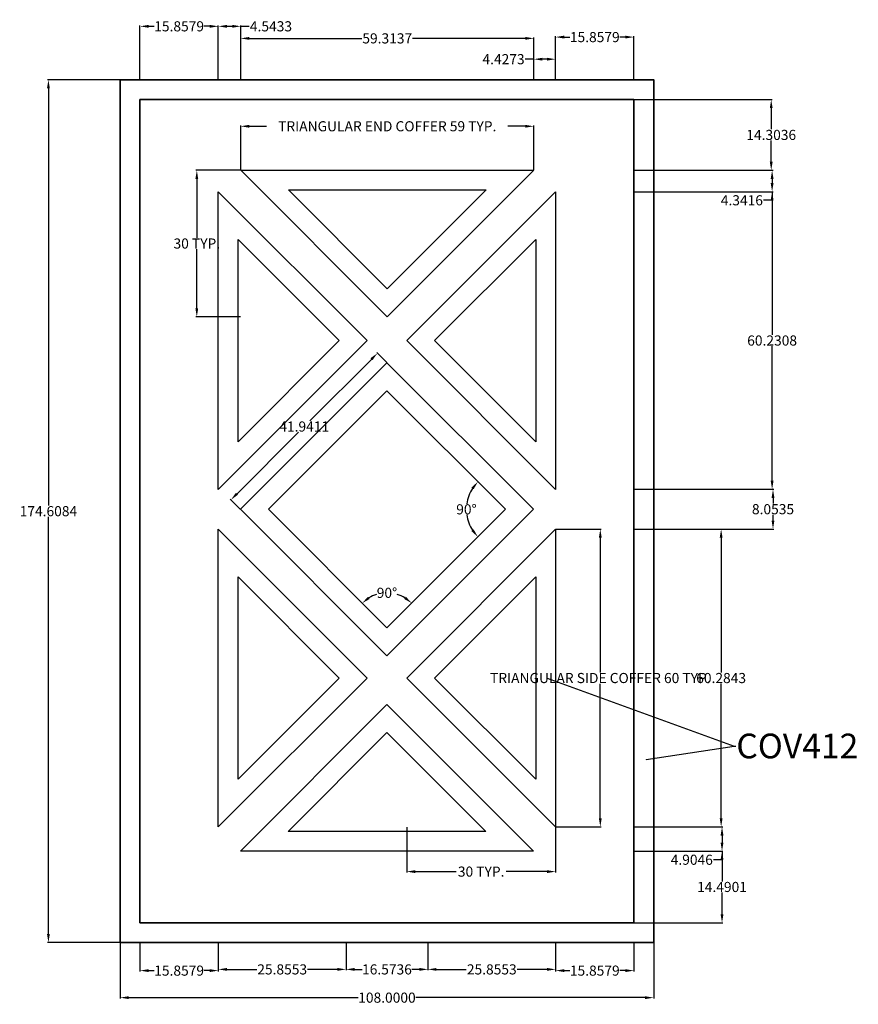
# Model space of a CAD drawing. Units: inches. Extents: x 854 to 1024, y 578 to 778.
import ezdxf
from ezdxf import colors
from ezdxf.entities.mleader import LeaderData, LeaderLine
from ezdxf.math import Vec2, Vec3

# ---------------------------------------------------------------- set-up
doc = ezdxf.new("R2010")
doc.units = ezdxf.units.IN
doc.header["$MEASUREMENT"] = 0
for name, color, linetype, lineweight in [('A-ANNO-DIMS', 2, 'Continuous', 18), ('A-ANNO-TEXT', 3, 'Continuous', 18), ('A-CLNG', 7, 'Continuous', 35), ('A-CLNG-COFR', 4, 'Continuous', 25)]:
    doc.layers.add(name, color=color, linetype=linetype, lineweight=lineweight)
doc.styles.get("Standard").update_dxf_attribs({"font": 'arial.ttf'})
doc.dimstyles.get("Standard").update_dxf_attribs({"dimtxt": 2.0485, "dimasz": 1.737, "dimexe": 0.18, "dimexo": 0.0625, "dimgap": 0.09, "dimtad": 0, "dimtih": 1, "dimtoh": 1, "dimdec": 4, "dimzin": 0, "dimdsep": 46, "dimtxsty": 'Standard', "dimcen": 0.09, "dimadec": 0, "dimazin": 0, "dimtfac": 1, "dimtdec": 4, "dimtofl": 0, "dimtmove": 0, "dimatfit": 3, "dimfxl": 1, "dimtolj": 1, "dimtzin": 0, "dimarcsym": 0})

# ---------------------------------------------------------------- blocks, each defined once
blk = doc.blocks.new('*D1')
at = {"layer": 'A-ANNO-DIMS', "color": 0, "lineweight": -2, "transparency": 16777216}
for start, end in [(147.6108, 171.7413), (188.2587, 212.3892)]:
    blk.add_arc((952.75, 678.63), 7.91, start, end, dxfattribs=at)
at = {"layer": 'A-ANNO-DIMS', "color": 0, "transparency": 16777216}
for points in [[(945.85, 683.05), (946.3, 682.69), (947.16, 684.23)], [(946.3, 674.58), (945.85, 674.22), (947.16, 673.04)]]:
    blk.add_solid(points, dxfattribs=at)
at = {"layer": 'Defpoints', "color": 0, "transparency": 16777216}
for p in [(928.75, 702.63), (945.11, 680.68), (952.75, 678.63), (952.75, 678.63), (928.75, 654.63)]:
    blk.add_point(p, dxfattribs=at)
at = {"layer": 'A-ANNO-DIMS', "color": 0, "transparency": 16777216, "insert": (944.84, 678.63), "char_height": 2.049, "attachment_point": 5}
blk.add_mtext('\\A1;90°', dxfattribs=at)
blk = doc.blocks.new('*D2')
at = {"layer": 'A-ANNO-DIMS', "color": 0, "lineweight": -2, "transparency": 16777216}
for start, end in [(107.2, 120.9465), (59.0535, 72.8)]:
    blk.add_arc((928.75, 654.63), 7.1, start, end, dxfattribs=at)
at = {"layer": 'A-ANNO-DIMS', "color": 0, "transparency": 16777216}
for points in [[(925.28, 660.5), (924.92, 660.95), (923.73, 659.65)], [(932.58, 660.95), (932.22, 660.5), (933.77, 659.65)]]:
    blk.add_solid(points, dxfattribs=at)
at = {"layer": 'Defpoints', "color": 0, "transparency": 16777216}
for p in [(904.75, 678.63), (952.75, 678.63), (930.59, 661.49), (928.75, 654.63), (928.75, 654.63)]:
    blk.add_point(p, dxfattribs=at)
at = {"layer": 'A-ANNO-DIMS', "color": 0, "transparency": 16777216, "insert": (928.75, 661.73), "char_height": 2.049, "attachment_point": 5}
blk.add_mtext('\\A1;90°', dxfattribs=at)
blk = doc.blocks.new('*D3')
at = {"layer": 'A-ANNO-DIMS', "color": 0, "lineweight": -2, "transparency": 16777216}
for p, q in [((928.71, 708.34), (926.7, 710.35)), ((925.6, 708.99), (913.13, 696.53)), ((898.4, 681.79), (910.86, 694.25)), ((899.05, 678.68), (897.04, 680.69))]:
    blk.add_line(p, q, dxfattribs=at)
at = {"layer": 'A-ANNO-DIMS', "color": 0, "transparency": 16777216}
for points in [[(925.39, 709.2), (925.8, 708.79), (926.82, 710.22)], [(898.19, 682), (898.6, 681.59), (897.17, 680.56)]]:
    blk.add_solid(points, dxfattribs=at)
at = {"layer": 'Defpoints', "color": 0, "transparency": 16777216}
for p in [(926.82, 710.22), (928.75, 708.29), (899.09, 678.63)]:
    blk.add_point(p, dxfattribs=at)
at = {"layer": 'A-ANNO-DIMS', "color": 0, "transparency": 16777216, "insert": (912, 695.39), "char_height": 2.0485, "attachment_point": 5}
blk.add_mtext('\\A1;41.9411', dxfattribs=at)
blk = doc.blocks.new('*D4')
at = {"layer": 'A-ANNO-DIMS', "color": 0, "lineweight": -2, "transparency": 16777216}
for p, q in [((874.75, 590.89), (874.75, 579.62)), ((982.75, 590.89), (982.75, 579.62)), ((876.49, 579.8), (922.92, 579.8)), ((981.01, 579.8), (934.58, 579.8))]:
    blk.add_line(p, q, dxfattribs=at)
at = {"layer": 'A-ANNO-DIMS', "color": 0, "transparency": 16777216}
for points in [[(876.49, 580.09), (876.49, 579.51), (874.75, 579.8)], [(981.01, 580.09), (981.01, 579.51), (982.75, 579.8)]]:
    blk.add_solid(points, dxfattribs=at)
at = {"layer": 'Defpoints', "color": 0, "transparency": 16777216}
for p in [(874.75, 590.96), (982.75, 590.96), (982.75, 579.8)]:
    blk.add_point(p, dxfattribs=at)
at = {"layer": 'A-ANNO-DIMS', "color": 0, "transparency": 16777216, "insert": (928.75, 579.8), "char_height": 2.0485, "attachment_point": 5}
blk.add_mtext('\\A1;108.0000', dxfattribs=at)
blk = doc.blocks.new('*D5')
at = {"layer": 'A-ANNO-DIMS', "color": 0, "lineweight": -2, "transparency": 16777216}
for p, q in [((874.69, 765.56), (860.04, 765.56)), ((860.22, 763.83), (860.22, 679.4)), ((860.22, 592.69), (860.22, 677.12)), ((874.69, 590.96), (860.04, 590.96))]:
    blk.add_line(p, q, dxfattribs=at)
at = {"layer": 'A-ANNO-DIMS', "color": 0, "transparency": 16777216}
for points in [[(859.93, 763.83), (860.51, 763.83), (860.22, 765.56)], [(859.93, 592.69), (860.51, 592.69), (860.22, 590.96)]]:
    blk.add_solid(points, dxfattribs=at)
at = {"layer": 'Defpoints', "color": 0, "transparency": 16777216}
for p in [(874.75, 765.56), (860.22, 590.96), (874.75, 590.96)]:
    blk.add_point(p, dxfattribs=at)
at = {"layer": 'A-ANNO-DIMS', "color": 0, "transparency": 16777216, "insert": (860.22, 678.26), "char_height": 2.0485, "attachment_point": 5}
blk.add_mtext('\\A1;174.6084', dxfattribs=at)
blk = doc.blocks.new('*D6')
at = {"layer": 'A-ANNO-DIMS', "color": 0, "lineweight": -2, "transparency": 16777216}
for p, q in [((878.75, 765.63), (878.75, 776.57)), ((880.49, 776.39), (881.64, 776.39)), ((892.87, 776.39), (891.72, 776.39)), ((894.61, 765.63), (894.61, 776.57))]:
    blk.add_line(p, q, dxfattribs=at)
at = {"layer": 'A-ANNO-DIMS', "color": 0, "transparency": 16777216}
for points in [[(880.49, 776.68), (880.49, 776.1), (878.75, 776.39)], [(892.87, 776.68), (892.87, 776.1), (894.61, 776.39)]]:
    blk.add_solid(points, dxfattribs=at)
at = {"layer": 'Defpoints', "color": 0, "transparency": 16777216}
for p in [(894.61, 776.39), (878.75, 765.56), (894.61, 765.56)]:
    blk.add_point(p, dxfattribs=at)
at = {"layer": 'A-ANNO-DIMS', "color": 0, "transparency": 16777216, "insert": (886.68, 776.39), "char_height": 2.0485, "attachment_point": 5}
blk.add_mtext('\\A1;15.8579', dxfattribs=at)
blk = doc.blocks.new('*D7')
at = {"layer": 'A-ANNO-DIMS', "color": 0, "lineweight": -2, "transparency": 16777216}
for p, q in [((894.61, 765.63), (894.61, 776.57)), ((896.35, 776.39), (897.42, 776.39)), ((899.15, 765.63), (899.15, 776.57)), ((899.15, 776.39), (900.89, 776.39))]:
    blk.add_line(p, q, dxfattribs=at)
at = {"layer": 'A-ANNO-DIMS', "color": 0, "transparency": 16777216}
for points in [[(896.35, 776.68), (896.35, 776.1), (894.61, 776.39)], [(897.42, 776.68), (897.42, 776.1), (899.15, 776.39)]]:
    blk.add_solid(points, dxfattribs=at)
at = {"layer": 'Defpoints', "color": 0, "transparency": 16777216}
for p in [(899.15, 776.39), (894.61, 765.56), (899.15, 765.56)]:
    blk.add_point(p, dxfattribs=at)
at = {"layer": 'A-ANNO-DIMS', "color": 0, "transparency": 16777216, "insert": (905.27, 776.39), "char_height": 2.049, "attachment_point": 5}
blk.add_mtext('\\A1;4.5433', dxfattribs=at)
blk = doc.blocks.new('*D8')
at = {"layer": 'A-ANNO-DIMS', "color": 0, "lineweight": -2, "transparency": 16777216}
for p, q in [((899.15, 765.63), (899.15, 774.13)), ((900.89, 773.95), (923.67, 773.95)), ((956.73, 773.95), (933.95, 773.95)), ((958.47, 765.63), (958.47, 774.13))]:
    blk.add_line(p, q, dxfattribs=at)
at = {"layer": 'A-ANNO-DIMS', "color": 0, "transparency": 16777216}
for points in [[(900.89, 774.24), (900.89, 773.66), (899.15, 773.95)], [(956.73, 774.24), (956.73, 773.66), (958.47, 773.95)]]:
    blk.add_solid(points, dxfattribs=at)
at = {"layer": 'Defpoints', "color": 0, "transparency": 16777216}
for p in [(958.47, 773.95), (899.15, 765.56), (958.47, 765.56)]:
    blk.add_point(p, dxfattribs=at)
at = {"layer": 'A-ANNO-DIMS', "color": 0, "transparency": 16777216, "insert": (928.81, 773.95), "char_height": 2.0485, "attachment_point": 5}
blk.add_mtext('\\A1;59.3137', dxfattribs=at)
blk = doc.blocks.new('*D9')
at = {"layer": 'A-ANNO-DIMS', "color": 0, "lineweight": -2, "transparency": 16777216}
for p, q in [((958.47, 769.74), (956.73, 769.74)), ((958.47, 765.63), (958.47, 769.92)), ((961.16, 769.74), (960.2, 769.74)), ((962.89, 765.63), (962.89, 769.92))]:
    blk.add_line(p, q, dxfattribs=at)
at = {"layer": 'A-ANNO-DIMS', "color": 0, "transparency": 16777216}
for points in [[(960.2, 770.02), (960.2, 769.45), (958.47, 769.74)], [(961.16, 770.02), (961.16, 769.45), (962.89, 769.74)]]:
    blk.add_solid(points, dxfattribs=at)
at = {"layer": 'Defpoints', "color": 0, "transparency": 16777216}
for p in [(958.47, 769.74), (958.47, 765.56), (962.89, 765.56)]:
    blk.add_point(p, dxfattribs=at)
at = {"layer": 'A-ANNO-DIMS', "color": 0, "transparency": 16777216, "insert": (952.35, 769.74), "char_height": 2.049, "attachment_point": 5}
blk.add_mtext('\\A1;4.4273', dxfattribs=at)
blk = doc.blocks.new('*D10')
at = {"layer": 'A-ANNO-DIMS', "color": 0, "lineweight": -2, "transparency": 16777216}
for p, q in [((962.89, 765.63), (962.89, 774.39)), ((964.63, 774.21), (965.78, 774.21)), ((977.01, 774.21), (975.87, 774.21)), ((978.75, 765.63), (978.75, 774.39))]:
    blk.add_line(p, q, dxfattribs=at)
at = {"layer": 'A-ANNO-DIMS', "color": 0, "transparency": 16777216}
for points in [[(964.63, 774.5), (964.63, 773.92), (962.89, 774.21)], [(977.01, 774.5), (977.01, 773.92), (978.75, 774.21)]]:
    blk.add_solid(points, dxfattribs=at)
at = {"layer": 'Defpoints', "color": 0, "transparency": 16777216}
for p in [(978.75, 774.21), (962.89, 765.56), (978.75, 765.56)]:
    blk.add_point(p, dxfattribs=at)
at = {"layer": 'A-ANNO-DIMS', "color": 0, "transparency": 16777216, "insert": (970.82, 774.21), "char_height": 2.0485, "attachment_point": 5}
blk.add_mtext('\\A1;15.8579', dxfattribs=at)
blk = doc.blocks.new('*D11')
at = {"layer": 'A-ANNO-DIMS', "color": 0, "lineweight": -2, "transparency": 16777216}
for p, q in [((878.75, 590.89), (878.75, 585.09)), ((894.61, 590.89), (894.61, 585.09)), ((880.49, 585.27), (881.64, 585.27)), ((892.87, 585.27), (891.72, 585.27))]:
    blk.add_line(p, q, dxfattribs=at)
at = {"layer": 'A-ANNO-DIMS', "color": 0, "transparency": 16777216}
for points in [[(880.49, 585.56), (880.49, 584.98), (878.75, 585.27)], [(892.87, 585.56), (892.87, 584.98), (894.61, 585.27)]]:
    blk.add_solid(points, dxfattribs=at)
at = {"layer": 'Defpoints', "color": 0, "transparency": 16777216}
for p in [(878.75, 590.96), (894.61, 590.96), (878.75, 585.27)]:
    blk.add_point(p, dxfattribs=at)
at = {"layer": 'A-ANNO-DIMS', "color": 0, "transparency": 16777216, "insert": (886.68, 585.27), "char_height": 2.0485, "attachment_point": 5}
blk.add_mtext('\\A1;15.8579', dxfattribs=at)
blk = doc.blocks.new('*D12')
at = {"layer": 'A-ANNO-DIMS', "color": 0, "lineweight": -2, "transparency": 16777216}
for p, q in [((894.61, 590.89), (894.61, 585.34)), ((920.46, 590.89), (920.46, 585.34)), ((896.35, 585.52), (902.38, 585.52)), ((918.73, 585.52), (912.69, 585.52))]:
    blk.add_line(p, q, dxfattribs=at)
at = {"layer": 'A-ANNO-DIMS', "color": 0, "transparency": 16777216}
for points in [[(896.35, 585.81), (896.35, 585.23), (894.61, 585.52)], [(918.73, 585.81), (918.73, 585.23), (920.46, 585.52)]]:
    blk.add_solid(points, dxfattribs=at)
at = {"layer": 'Defpoints', "color": 0, "transparency": 16777216}
for p in [(894.61, 590.96), (920.46, 590.96), (920.46, 585.52)]:
    blk.add_point(p, dxfattribs=at)
at = {"layer": 'A-ANNO-DIMS', "color": 0, "transparency": 16777216, "insert": (907.54, 585.52), "char_height": 2.0485, "attachment_point": 5}
blk.add_mtext('\\A1;25.8553', dxfattribs=at)
blk = doc.blocks.new('*D14')
at = {"layer": 'A-ANNO-DIMS', "color": 0, "lineweight": -2, "transparency": 16777216}
for p, q in [((962.89, 590.89), (962.89, 585.09)), ((978.75, 590.89), (978.75, 585.09)), ((964.63, 585.27), (965.78, 585.27)), ((977.01, 585.27), (975.87, 585.27))]:
    blk.add_line(p, q, dxfattribs=at)
at = {"layer": 'A-ANNO-DIMS', "color": 0, "transparency": 16777216}
for points in [[(964.63, 585.56), (964.63, 584.98), (962.89, 585.27)], [(977.01, 585.56), (977.01, 584.98), (978.75, 585.27)]]:
    blk.add_solid(points, dxfattribs=at)
at = {"layer": 'Defpoints', "color": 0, "transparency": 16777216}
for p in [(962.89, 590.96), (978.75, 590.96), (978.75, 585.27)]:
    blk.add_point(p, dxfattribs=at)
at = {"layer": 'A-ANNO-DIMS', "color": 0, "transparency": 16777216, "insert": (970.82, 585.27), "char_height": 2.0485, "attachment_point": 5}
blk.add_mtext('\\A1;15.8579', dxfattribs=at)
blk = doc.blocks.new('*D13')
at = {"layer": 'A-ANNO-DIMS', "color": 0, "lineweight": -2, "transparency": 16777216}
for p, q in [((937.04, 590.89), (937.04, 585.34)), ((962.89, 590.89), (962.89, 585.34)), ((938.77, 585.52), (944.81, 585.52)), ((961.16, 585.52), (955.12, 585.52))]:
    blk.add_line(p, q, dxfattribs=at)
at = {"layer": 'A-ANNO-DIMS', "color": 0, "transparency": 16777216}
for points in [[(938.77, 585.81), (938.77, 585.23), (937.04, 585.52)], [(961.16, 585.81), (961.16, 585.23), (962.89, 585.52)]]:
    blk.add_solid(points, dxfattribs=at)
at = {"layer": 'Defpoints', "color": 0, "transparency": 16777216}
for p in [(937.04, 590.96), (962.89, 590.96), (937.04, 585.52)]:
    blk.add_point(p, dxfattribs=at)
at = {"layer": 'A-ANNO-DIMS', "color": 0, "transparency": 16777216, "insert": (949.97, 585.52), "char_height": 2.0485, "attachment_point": 5}
blk.add_mtext('\\A1;25.8553', dxfattribs=at)
blk = doc.blocks.new('*D15')
at = {"layer": 'A-ANNO-DIMS', "color": 0, "lineweight": -2, "transparency": 16777216}
for p, q in [((920.46, 590.89), (920.46, 585.34)), ((937.04, 590.89), (937.04, 585.34)), ((922.2, 585.52), (923.71, 585.52)), ((935.3, 585.52), (933.79, 585.52))]:
    blk.add_line(p, q, dxfattribs=at)
at = {"layer": 'A-ANNO-DIMS', "color": 0, "transparency": 16777216}
for points in [[(922.2, 585.81), (922.2, 585.23), (920.46, 585.52)], [(935.3, 585.81), (935.3, 585.23), (937.04, 585.52)]]:
    blk.add_solid(points, dxfattribs=at)
at = {"layer": 'Defpoints', "color": 0, "transparency": 16777216}
for p in [(920.46, 590.96), (937.04, 590.96), (937.04, 585.52)]:
    blk.add_point(p, dxfattribs=at)
at = {"layer": 'A-ANNO-DIMS', "color": 0, "transparency": 16777216, "insert": (928.75, 585.52), "char_height": 2.0485, "attachment_point": 5}
blk.add_mtext('\\A1;16.5736', dxfattribs=at)
blk = doc.blocks.new('*D16')
at = {"layer": 'A-ANNO-DIMS', "color": 0, "lineweight": -2, "transparency": 16777216}
for p, q in [((978.81, 761.56), (1006.72, 761.56)), ((1006.54, 759.83), (1006.54, 755.55)), ((1006.54, 749), (1006.54, 753.28)), ((979.95, 747.26), (1006.72, 747.26))]:
    blk.add_line(p, q, dxfattribs=at)
at = {"layer": 'A-ANNO-DIMS', "color": 0, "transparency": 16777216}
for points in [[(1006.25, 759.83), (1006.83, 759.83), (1006.54, 761.56)], [(1006.25, 749), (1006.83, 749), (1006.54, 747.26)]]:
    blk.add_solid(points, dxfattribs=at)
at = {"layer": 'Defpoints', "color": 0, "transparency": 16777216}
for p in [(978.75, 761.56), (979.89, 747.26), (1006.54, 747.26)]:
    blk.add_point(p, dxfattribs=at)
at = {"layer": 'A-ANNO-DIMS', "color": 0, "transparency": 16777216, "insert": (1006.54, 754.41), "char_height": 2.0485, "attachment_point": 5}
blk.add_mtext('\\A1;14.3036', dxfattribs=at)
blk = doc.blocks.new('*D17')
at = {"layer": 'A-ANNO-DIMS', "color": 0, "lineweight": -2, "transparency": 16777216}
for p, q in [((978.81, 747.26), (1006.9, 747.26)), ((1006.72, 745.52), (1006.72, 744.66)), ((978.81, 742.92), (1006.9, 742.92)), ((1006.72, 742.92), (1006.72, 741.18)), ((1006.72, 741.18), (1004.98, 741.18))]:
    blk.add_line(p, q, dxfattribs=at)
at = {"layer": 'A-ANNO-DIMS', "color": 0, "transparency": 16777216}
for points in [[(1006.43, 745.52), (1007.01, 745.52), (1006.72, 747.26)], [(1006.43, 744.66), (1007.01, 744.66), (1006.72, 742.92)]]:
    blk.add_solid(points, dxfattribs=at)
at = {"layer": 'Defpoints', "color": 0, "transparency": 16777216}
for p in [(978.75, 747.26), (978.75, 742.92), (1006.72, 742.92)]:
    blk.add_point(p, dxfattribs=at)
at = {"layer": 'A-ANNO-DIMS', "color": 0, "transparency": 16777216, "insert": (1000.6, 741.18), "char_height": 2.049, "attachment_point": 5}
blk.add_mtext('\\A1;4.3416', dxfattribs=at)
blk = doc.blocks.new('*D18')
at = {"layer": 'A-ANNO-DIMS', "color": 0, "lineweight": -2, "transparency": 16777216}
for p, q in [((978.81, 742.92), (1006.9, 742.92)), ((1006.72, 741.18), (1006.72, 713.94)), ((1006.72, 684.43), (1006.72, 711.67)), ((978.81, 682.69), (1006.9, 682.69))]:
    blk.add_line(p, q, dxfattribs=at)
at = {"layer": 'A-ANNO-DIMS', "color": 0, "transparency": 16777216}
for points in [[(1006.43, 741.18), (1007.01, 741.18), (1006.72, 742.92)], [(1006.43, 684.43), (1007.01, 684.43), (1006.72, 682.69)]]:
    blk.add_solid(points, dxfattribs=at)
at = {"layer": 'Defpoints', "color": 0, "transparency": 16777216}
for p in [(978.75, 742.92), (978.75, 682.69), (1006.72, 682.69)]:
    blk.add_point(p, dxfattribs=at)
at = {"layer": 'A-ANNO-DIMS', "color": 0, "transparency": 16777216, "insert": (1006.72, 712.8), "char_height": 2.0485, "attachment_point": 5}
blk.add_mtext('\\A1;60.2308', dxfattribs=at)
blk = doc.blocks.new('*D19')
at = {"layer": 'A-ANNO-DIMS', "color": 0, "lineweight": -2, "transparency": 16777216}
for p, q in [((978.81, 682.69), (1007.08, 682.69)), ((1006.9, 680.95), (1006.9, 679.8)), ((1006.9, 676.37), (1006.9, 677.52)), ((978.81, 674.63), (1007.08, 674.63))]:
    blk.add_line(p, q, dxfattribs=at)
at = {"layer": 'A-ANNO-DIMS', "color": 0, "transparency": 16777216}
for points in [[(1006.61, 680.95), (1007.19, 680.95), (1006.9, 682.69)], [(1006.61, 676.37), (1007.19, 676.37), (1006.9, 674.63)]]:
    blk.add_solid(points, dxfattribs=at)
at = {"layer": 'Defpoints', "color": 0, "transparency": 16777216}
for p in [(978.75, 682.69), (978.75, 674.63), (1006.9, 674.63)]:
    blk.add_point(p, dxfattribs=at)
at = {"layer": 'A-ANNO-DIMS', "color": 0, "transparency": 16777216, "insert": (1006.9, 678.66), "char_height": 2.049, "attachment_point": 5}
blk.add_mtext('\\A1;8.0535', dxfattribs=at)
blk = doc.blocks.new('*D20')
at = {"layer": 'A-ANNO-DIMS', "color": 0, "lineweight": -2, "transparency": 16777216}
for p, q in [((978.81, 674.63), (996.58, 674.63)), ((996.4, 672.9), (996.4, 645.63)), ((996.4, 616.09), (996.4, 643.36)), ((978.81, 614.35), (996.58, 614.35))]:
    blk.add_line(p, q, dxfattribs=at)
at = {"layer": 'A-ANNO-DIMS', "color": 0, "transparency": 16777216}
for points in [[(996.11, 672.9), (996.69, 672.9), (996.4, 674.63)], [(996.11, 616.09), (996.69, 616.09), (996.4, 614.35)]]:
    blk.add_solid(points, dxfattribs=at)
at = {"layer": 'Defpoints', "color": 0, "transparency": 16777216}
for p in [(978.75, 674.63), (978.75, 614.35), (996.4, 614.35)]:
    blk.add_point(p, dxfattribs=at)
at = {"layer": 'A-ANNO-DIMS', "color": 0, "transparency": 16777216, "insert": (996.4, 644.49), "char_height": 2.0485, "attachment_point": 5}
blk.add_mtext('\\A1;60.2843', dxfattribs=at)
blk = doc.blocks.new('*D21')
at = {"layer": 'A-ANNO-DIMS', "color": 0, "lineweight": -2, "transparency": 16777216}
for p, q in [((978.81, 614.35), (996.76, 614.35)), ((996.58, 612.61), (996.58, 611.18)), ((978.81, 609.45), (996.76, 609.45)), ((996.58, 609.45), (996.58, 607.71)), ((996.58, 607.71), (994.84, 607.71))]:
    blk.add_line(p, q, dxfattribs=at)
at = {"layer": 'A-ANNO-DIMS', "color": 0, "transparency": 16777216}
for points in [[(996.29, 612.61), (996.87, 612.61), (996.58, 614.35)], [(996.29, 611.18), (996.87, 611.18), (996.58, 609.45)]]:
    blk.add_solid(points, dxfattribs=at)
at = {"layer": 'Defpoints', "color": 0, "transparency": 16777216}
for p in [(978.75, 614.35), (978.75, 609.45), (996.58, 609.45)]:
    blk.add_point(p, dxfattribs=at)
at = {"layer": 'A-ANNO-DIMS', "color": 0, "transparency": 16777216, "insert": (990.46, 607.71), "char_height": 2.049, "attachment_point": 5}
blk.add_mtext('\\A1;4.9046', dxfattribs=at)
blk = doc.blocks.new('*D22')
at = {"layer": 'A-ANNO-DIMS', "color": 0, "lineweight": -2, "transparency": 16777216}
for p, q in [((978.81, 609.45), (996.76, 609.45)), ((996.58, 607.71), (996.58, 603.34)), ((996.58, 596.69), (996.58, 601.06)), ((978.81, 594.96), (996.76, 594.96))]:
    blk.add_line(p, q, dxfattribs=at)
at = {"layer": 'A-ANNO-DIMS', "color": 0, "transparency": 16777216}
for points in [[(996.29, 607.71), (996.87, 607.71), (996.58, 609.45)], [(996.29, 596.69), (996.87, 596.69), (996.58, 594.96)]]:
    blk.add_solid(points, dxfattribs=at)
at = {"layer": 'Defpoints', "color": 0, "transparency": 16777216}
for p in [(978.75, 609.45), (978.75, 594.96), (996.58, 594.96)]:
    blk.add_point(p, dxfattribs=at)
at = {"layer": 'A-ANNO-DIMS', "color": 0, "transparency": 16777216, "insert": (996.58, 602.2), "char_height": 2.0485, "attachment_point": 5}
blk.add_mtext('\\A1;14.4901', dxfattribs=at)
blk = doc.blocks.new('COFFER-TRI-SIDE')
for p, q in [((0, 0), (0, 60.28)), ((4, 9.66), (4, 50.63))]:
    blk.add_line(p, q)
for points in [[(0, 60.28), (30.14, 30.14)], [(4, 50.63), (24.49, 30.14)], [(0, 0), (30.14, 30.14)], [(4, 9.66), (24.49, 30.14)]]:
    blk.add_lwpolyline(points)
blk = doc.blocks.new('COFFER-TRI-END')
for p, q in [((0, 29.66), (59.31, 29.66)), ((9.66, 25.66), (49.66, 25.66))]:
    blk.add_line(p, q)
for points in [[(0, 29.66), (29.66, 0), (59.31, 29.66)], [(9.66, 25.66), (29.66, 5.66), (49.66, 25.66)]]:
    blk.add_lwpolyline(points)
blk = doc.blocks.new('*D25')
at = {"layer": 'A-ANNO-DIMS', "color": 0, "lineweight": -2, "transparency": 16777216}
for p, q in [((962.96, 674.63), (972.12, 674.63)), ((971.94, 672.9), (971.94, 645.64)), ((971.94, 616.09), (971.94, 643.34)), ((962.96, 614.35), (972.12, 614.35))]:
    blk.add_line(p, q, dxfattribs=at)
at = {"layer": 'A-ANNO-DIMS', "color": 0, "transparency": 16777216}
for points in [[(971.65, 672.9), (972.23, 672.9), (971.94, 674.63)], [(971.65, 616.09), (972.23, 616.09), (971.94, 614.35)]]:
    blk.add_solid(points, dxfattribs=at)
at = {"layer": 'Defpoints', "color": 0, "transparency": 16777216}
for p in [(962.89, 674.63), (962.89, 614.35), (971.94, 614.35)]:
    blk.add_point(p, dxfattribs=at)
at = {"layer": 'A-ANNO-DIMS', "color": 0, "transparency": 16777216, "insert": (971.94, 644.49), "char_height": 2.0485, "attachment_point": 5}
blk.add_mtext('\\A1;TRIANGULAR SIDE COFFER 60 TYP.', dxfattribs=at)
blk = doc.blocks.new('*D26')
at = {"layer": 'A-ANNO-DIMS', "color": 0, "lineweight": -2, "transparency": 16777216}
for p, q in [((932.75, 614.29), (932.75, 605.13)), ((962.89, 614.29), (962.89, 605.13)), ((934.49, 605.31), (942.75, 605.31)), ((961.16, 605.31), (952.9, 605.31))]:
    blk.add_line(p, q, dxfattribs=at)
at = {"layer": 'A-ANNO-DIMS', "color": 0, "transparency": 16777216}
for points in [[(934.49, 605.6), (934.49, 605.02), (932.75, 605.31)], [(961.16, 605.6), (961.16, 605.02), (962.89, 605.31)]]:
    blk.add_solid(points, dxfattribs=at)
at = {"layer": 'Defpoints', "color": 0, "transparency": 16777216}
for p in [(932.75, 614.35), (962.89, 614.35), (932.75, 605.31)]:
    blk.add_point(p, dxfattribs=at)
at = {"layer": 'A-ANNO-DIMS', "color": 0, "transparency": 16777216, "insert": (947.82, 605.31), "char_height": 2.0485, "attachment_point": 5}
blk.add_mtext('\\A1;30 TYP.', dxfattribs=at)
blk = doc.blocks.new('*D27')
at = {"layer": 'A-ANNO-DIMS', "color": 0, "lineweight": -2, "transparency": 16777216}
for p, q in [((899.15, 747.32), (899.15, 756.34)), ((900.89, 756.16), (904.39, 756.16)), ((956.73, 756.16), (953.23, 756.16)), ((958.47, 747.32), (958.47, 756.34))]:
    blk.add_line(p, q, dxfattribs=at)
at = {"layer": 'A-ANNO-DIMS', "color": 0, "transparency": 16777216}
for points in [[(900.89, 756.45), (900.89, 755.87), (899.15, 756.16)], [(956.73, 756.45), (956.73, 755.87), (958.47, 756.16)]]:
    blk.add_solid(points, dxfattribs=at)
at = {"layer": 'Defpoints', "color": 0, "transparency": 16777216}
for p in [(958.47, 756.16), (899.15, 747.26), (958.47, 747.26)]:
    blk.add_point(p, dxfattribs=at)
at = {"layer": 'A-ANNO-DIMS', "color": 0, "transparency": 16777216, "insert": (928.81, 756.16), "char_height": 2.0485, "attachment_point": 5}
blk.add_mtext('\\A1;TRIANGULAR END COFFER 59 TYP.', dxfattribs=at)
blk = doc.blocks.new('*D28')
at = {"layer": 'A-ANNO-DIMS', "color": 0, "lineweight": -2, "transparency": 16777216}
for p, q in [((899.09, 747.26), (890.08, 747.26)), ((890.26, 745.52), (890.26, 733.57)), ((890.26, 719.34), (890.26, 731.3)), ((899.09, 717.6), (890.08, 717.6))]:
    blk.add_line(p, q, dxfattribs=at)
at = {"layer": 'A-ANNO-DIMS', "color": 0, "transparency": 16777216}
for points in [[(889.97, 745.52), (890.54, 745.52), (890.26, 747.26)], [(889.97, 719.34), (890.54, 719.34), (890.26, 717.6)]]:
    blk.add_solid(points, dxfattribs=at)
at = {"layer": 'Defpoints', "color": 0, "transparency": 16777216}
for p in [(890.26, 747.26), (899.15, 747.26), (899.15, 717.6)]:
    blk.add_point(p, dxfattribs=at)
at = {"layer": 'A-ANNO-DIMS', "color": 0, "transparency": 16777216, "insert": (890.26, 732.43), "char_height": 2.0485, "attachment_point": 5}
blk.add_mtext('\\A1;30 TYP.', dxfattribs=at)

msp = doc.modelspace()

# ---------------------------------------------------------------- linework, layer by layer
at = {"layer": 'A-CLNG'}
for points in [[(874.75116, 765.56427), (982.75116, 765.56427), (982.75116, 590.95583), (874.75116, 590.95583)], [(878.75116, 761.56427), (978.75116, 761.56427), (978.75116, 594.95583), (878.75116, 594.95583)]]:
    msp.add_lwpolyline(points, close=True, dxfattribs=at)
at = {"layer": 'A-CLNG-COFR'}
for points in [[(928.75116, 648.97798), (899.09431, 678.63484), (928.75116, 708.29169), (958.40802, 678.63484)], [(928.75116, 654.63484), (904.75116, 678.63484), (928.75116, 702.63484), (952.75116, 678.63484)]]:
    msp.add_lwpolyline(points, close=True, dxfattribs=at)

# ---------------------------------------------------------------- block references
for name, p in [('COFFER-TRI-END', (899.152, 717.604)), ('COFFER-TRI-SIDE', (894.609, 682.635)), ('COFFER-TRI-SIDE', (894.609, 614.35073))]:
    msp.add_blockref(name, p, dxfattribs=at)
at = {"layer": 'A-CLNG-COFR', "rotation": 180}
for name, p in [('COFFER-TRI-SIDE', (962.89333, 742.91895)), ('COFFER-TRI-SIDE', (962.89333, 674.63468)), ('COFFER-TRI-END', (958.40831, 639.10264))]:
    msp.add_blockref(name, p, dxfattribs=at)

# ---------------------------------------------------------------- dimensions: what is measured, and where the dimension line sits
at = {"layer": 'A-ANNO-DIMS'}
for base, p1, p2, picture, middle in [((894.60903, 776.38685), (878.75116, 765.56427), (894.60903, 765.56427), '*D6', (886.6801, 776.38685)), ((899.1523, 776.38685), (894.60903, 765.56427), (899.1523, 765.56427), '*D7', (905.27262, 776.38685)), ((958.466, 773.95394), (899.1523, 765.56427), (958.466, 765.56427), '*D8', (928.80915, 773.95394)), ((978.75116, 774.20963), (962.8933, 765.56427), (978.75116, 765.56427), '*D10', (970.82223, 774.20963)), ((958.466, 769.73524), (962.8933, 765.56427), (958.466, 765.56427), '*D9', (952.34568, 769.73524)), ((982.75116, 579.79681), (874.75116, 590.95583), (982.75116, 590.95583), '*D4', (928.75116, 579.79681)), ((878.75116, 585.26947), (894.60903, 590.95583), (878.75116, 590.95583), '*D11', (886.6801, 585.26947)), ((920.46436, 585.52301), (894.60903, 590.95583), (920.46436, 590.95583), '*D12', (907.53669, 585.52301)), ((937.03797, 585.52301), (920.46436, 590.95583), (937.03797, 590.95583), '*D15', (928.75116, 585.52301))]:
    dim = msp.add_linear_dim(base=base, p1=p1, p2=p2, dimstyle='Standard', override={"dimclrd": 0, "dimclre": 0, "dimclrt": 0}, dxfattribs=at)
    dim.commit()
    dim.dimension.update_dxf_attribs({"geometry": picture, "text_midpoint": middle})
for base, p1, p2, angle, picture, middle in [((860.21891, 590.95583), (874.75116, 765.56427), (874.75116, 590.95583), 90, '*D5', (860.21891, 678.26005)), ((1006.53662, 747.26071), (978.75116, 761.56427), (979.88665, 747.26071), 90, '*D16', (1006.53662, 754.41249)), ((1006.71662, 742.91911), (978.75116, 747.26071), (978.75116, 742.91911), 90, '*D17', (1000.59699, 741.18211)), ((1006.71662, 682.68833), (978.75116, 742.91911), (978.75116, 682.68833), 90, '*D18', (1006.71662, 712.80372)), ((1006.89662, 674.63484), (978.75116, 682.68833), (978.75116, 674.63484), 90, '*D19', (1006.89662, 678.66159)), ((996.40086, 614.35057), (978.75116, 674.63484), (978.75116, 614.35057), 90, '*D20', (996.40086, 644.4927)), ((996.58086, 609.44593), (978.75116, 614.35057), (978.75116, 609.44593), 90, '*D21', (990.46124, 607.70893)), ((996.58086, 594.95583), (978.75116, 609.44593), (978.75116, 594.95583), 90, '*D22', (996.58086, 602.20088)), ((937.03797, 585.52301), (962.8933, 590.95583), (937.03797, 590.95583), 180, '*D13', (949.96563, 585.52301)), ((978.75116, 585.26947), (962.8933, 590.95583), (978.75116, 590.95583), 180, '*D14', (970.82223, 585.26947))]:
    dim = msp.add_linear_dim(base=base, p1=p1, p2=p2, angle=angle, dimstyle='Standard', override={"dimclrd": 0, "dimclre": 0, "dimclrt": 0}, dxfattribs=at)
    dim.commit()
    dim.dimension.update_dxf_attribs({"geometry": picture, "text_midpoint": middle})
dim = msp.add_linear_dim(base=(958.466, 756.15777), p1=(899.1523, 747.26071), p2=(958.466, 747.26071), text='TRIANGULAR END COFFER <> TYP.', dimstyle='Standard', override={"dimdec": 0, "dimlfac": 1, "dimrnd": 0, "dimzin": 0, "dimdsep": 46, "dimlunit": 2}, dxfattribs=at)
dim.commit()
dim.dimension.update_dxf_attribs({"geometry": '*D27', "text_midpoint": (928.80915, 756.15777)})
for base, p1, p2, angle, text, picture, middle in [((890.25524, 747.26071), (899.1523, 717.60386), (899.1523, 747.26071), 90, '<> TYP.', '*D28', (890.25524, 732.43228)), ((971.93594, 614.35057), (962.8933, 674.63484), (962.8933, 614.35057), 270, 'TRIANGULAR SIDE COFFER <> TYP.', '*D25', (971.93594, 644.4927)), ((932.75116, 605.30793), (962.8933, 614.35057), (932.75116, 614.35057), 180, '<> TYP.', '*D26', (947.82223, 605.30793))]:
    dim = msp.add_linear_dim(base=base, p1=p1, p2=p2, angle=angle, text=text, dimstyle='Standard', override={"dimdec": 0, "dimlfac": 1, "dimrnd": 0, "dimzin": 0, "dimdsep": 46, "dimlunit": 2}, dxfattribs=at)
    dim.commit()
    dim.dimension.update_dxf_attribs({"geometry": picture, "text_midpoint": middle})
dim = msp.add_aligned_dim(p1=(899.09431, 678.63484), p2=(928.75116, 708.29169), distance=2.72563, dimstyle='Standard', override={"dimclrd": 0, "dimclre": 0, "dimclrt": 0}, dxfattribs=at)
dim.commit()
dim.dimension.update_dxf_attribs({"geometry": '*D3', "text_midpoint": (911.99542, 695.39058)})
for base, line2, picture, middle in [((945.11277, 680.68154), ((928.75116, 702.63484), (952.75116, 678.63484)), '*D1', (944.84331, 678.63484)), ((930.58865, 661.49242), ((928.75116, 654.63484), (904.75116, 678.63484)), '*D2', (928.75116, 661.73433))]:
    dim = msp.add_angular_dim_2l(base=base, line1=((952.75116, 678.63484), (928.75116, 654.63484)), line2=line2, dimstyle='Standard', override={"dimclrd": 0, "dimclre": 0, "dimclrt": 0}, dxfattribs=at)
    dim.commit()
    dim.dimension.update_dxf_attribs({"geometry": picture, "text_midpoint": middle})

# ---------------------------------------------------------------- leaders
at = {"layer": 'A-ANNO-TEXT'}
ml = msp.add_multileader_mtext('Standard', dxfattribs=at)
ml.set_content('COV412', color=256)
ml.set_leader_properties()
ml.build(insert=Vec2(0, 0))
ml.multileader.update_dxf_attribs({"dogleg_length": 0.36, "arrow_head_size": 0.18})
ctx = ml.context
ctx.base_point, ctx.char_height, ctx.arrow_head_size, ctx.landing_gap_size, ctx.plane_origin = Vec3(999.38586, 630.69539), 5, 0.18, 0.09, Vec3(961.03301, 644.4927)
notes = []
notes.append((ctx, [(0, (1, 1, 0), (999.02586, 630.69539), (1, 0), 0.36, [(0, [(961.03301, 644.4927)], 0, []), (1, [(981.03155, 627.98219)], 0, [])])]))
ctx.mtext.insert, ctx.mtext.flow_direction = Vec3(999.47586, 633.23802), 5
for ctx, leaders in notes:
    for number, flags, end, landing, length, lines in leaders:
        leader = LeaderData()
        leader.index, (leader.has_last_leader_line, leader.has_dogleg_vector, leader.attachment_direction) = number, flags
        leader.last_leader_point, leader.dogleg_vector, leader.dogleg_length = Vec3(end), Vec3(landing), length
        for number, points, colour, breaks in lines:
            line = LeaderLine()
            line.index, line.vertices, line.color, line.breaks = number, Vec3.list(points), colors.encode_raw_color(colour), breaks
            leader.lines.append(line)
        ctx.leaders.append(leader)

doc.saveas('drawing.dxf')
